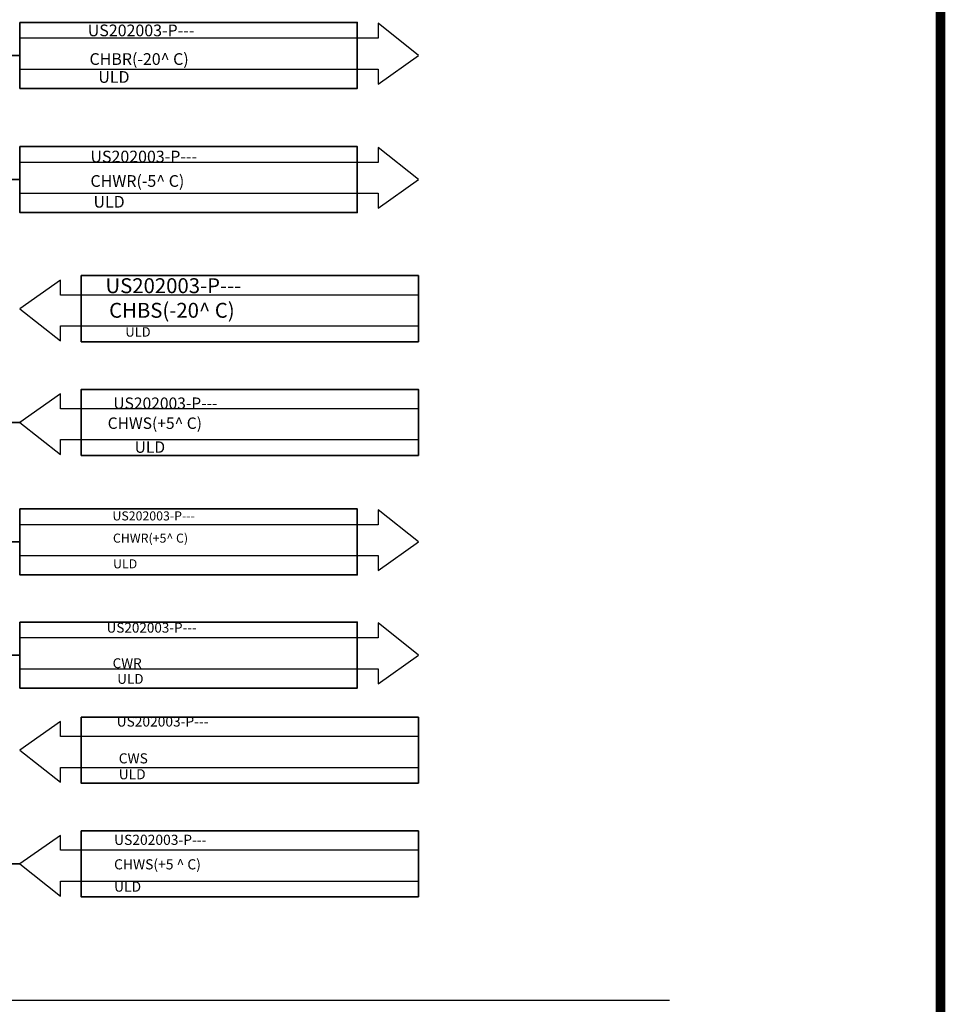
# Model space of a CAD drawing. Units: millimetres. Extents: x 353872 to 441597, y 126154 to 187356.
# Tile 27 of 28: x 426416 to 440911, y 157042 to 172470. Entities that reach past the tile are written whole.
import ezdxf

# ---------------------------------------------------------------- set-up
doc = ezdxf.new("R2010")
doc.units = ezdxf.units.MM
doc.linetypes.add('ACAD_ISO02W100', pattern=[15, 12, -3])
for name, color, linetype, lineweight in [('P-ANNO-TEXT', 7, 'Continuous', 25), ('P-ANNO-TTLB', 7, 'Continuous', 25), ('P-BNDY', 4, 'ACAD_ISO02W100', 25), ('P-EQPM', 5, 'Continuous', 35), ('P-PIPE', 3, 'Continuous', 35)]:
    doc.layers.add(name, color=color, linetype=linetype, lineweight=lineweight)
doc.styles.get("Standard").update_dxf_attribs({"font": 'arial.ttf'})

msp = doc.modelspace()

# ---------------------------------------------------------------- linework, layer by layer
at = {"layer": 'P-ANNO-TTLB', "const_width": 152.43}
msp.add_lwpolyline([(353948.03, 187280.05), (353948.03, 126916.34), (440835.19, 126916.34), (440835.19, 187280.05)], close=True, dxfattribs=at)
at = {"layer": 'P-ANNO-TTLB'}
for points in [[(426420.76, 171696.11), (432027.57, 171696.11), (432027.57, 171462.13), (432660.97, 171910.2), (432027.57, 172413.25), (432027.57, 172179.27), (426420.76, 172179.27)], [(426420.76, 169750.61), (432027.57, 169750.61), (432027.57, 169516.63), (432660.97, 169964.7), (432027.57, 170467.75), (432027.57, 170233.77), (426420.76, 170233.77)], [(432660.97, 168155.85), (427054.17, 168155.85), (427054.17, 168389.83), (426420.76, 167941.76), (427054.17, 167438.72), (427054.17, 167672.7), (432660.97, 167672.7)], [(432660.97, 166374.26), (427054.17, 166374.26), (427054.17, 166608.24), (426420.76, 166160.17), (427054.17, 165657.12), (427054.17, 165891.1), (432660.97, 165891.1)], [(426420.76, 164072.64), (432027.57, 164072.64), (432027.57, 163838.66), (432660.97, 164286.73), (432027.57, 164789.77), (432027.57, 164555.79), (426420.76, 164555.79)], [(426420.76, 162300.1), (432027.57, 162300.1), (432027.57, 162066.12), (432660.97, 162514.19), (432027.57, 163017.23), (432027.57, 162783.25), (426420.76, 162783.25)], [(432660.97, 161237.58), (427054.17, 161237.58), (427054.17, 161471.56), (426420.76, 161023.49), (427054.17, 160520.45), (427054.17, 160754.43), (432660.97, 160754.43)], [(432660.97, 159455.98), (427054.17, 159455.98), (427054.17, 159689.96), (426420.76, 159241.9), (427054.17, 158738.85), (427054.17, 158972.83), (432660.97, 158972.83)]]:
    msp.add_lwpolyline(points, dxfattribs=at)
at = {"layer": 'P-BNDY'}
msp.add_line((436591, 157104.68), (386532.91, 157104.68), dxfattribs=at)
at = {"layer": 'P-EQPM'}
for points in [[(426420.76, 172427.81), (431701.74, 172427.81), (431701.74, 171392.59), (426420.76, 171392.59)], [(426420.76, 170482.31), (431701.74, 170482.31), (431701.74, 169447.09), (426420.76, 169447.09)], [(432660.97, 167424.15), (427380, 167424.15), (427380, 168459.38), (432660.97, 168459.38)], [(432660.97, 165642.56), (427380, 165642.56), (427380, 166677.78), (432660.97, 166677.78)], [(426420.76, 164804.34), (431701.74, 164804.34), (431701.74, 163769.11), (426420.76, 163769.11)], [(426420.76, 163031.8), (431701.74, 163031.8), (431701.74, 161996.57), (426420.76, 161996.57)], [(432660.97, 160505.88), (427380, 160505.88), (427380, 161541.1), (432660.97, 161541.1)], [(432660.97, 158724.28), (427380, 158724.28), (427380, 159759.51), (432660.97, 159759.51)]]:
    msp.add_lwpolyline(points, close=True, dxfattribs=at)
at = {"layer": 'P-PIPE'}
for p, q in [((426420.76, 171910.2), (422379.04, 171907.06)), ((426420.76, 169964.7), (422379.04, 169964.7)), ((426439.3, 166160.17), (422437.83, 166160.17)), ((426420.76, 164286.73), (423379.37, 164286.73)), ((426420.76, 162514.19), (422688.58, 162514.19)), ((426420.76, 159241.9), (423545.52, 159241.9))]:
    msp.add_line(p, q, dxfattribs=at)

# ---------------------------------------------------------------- texts
at = {"layer": 'P-ANNO-TEXT'}
for s, height, p in [('US202003-P---', 183.3994, (427482.35, 172210.16)), ('CHBR(-20^  C)', 183.3994, (427509.64, 171761.64)), ('ULD', 183.399, (427647.52, 171480.84)), ('US202003-P---', 183.3994, (427524.22, 170233.77)), ('CHWR(-5^  C)', 183.3994, (427524.22, 169850.86)), ('ULD', 183.399, (427571.52, 169525.21)), ('US202003-P---', 233.6464, (427759.36, 168185.37)), ('CHBS(-20^  C)', 233.6464, (427816.34, 167799.73)), ('ULD', 148.533, (428070.7, 167503.59)), ('US202003-P---', 179.169, (427882.43, 166371.24)), ('CHWS(+5^  C)', 179.169, (427793.74, 166058.16)), ('ULD', 179.169, (428216.26, 165683.64)), ('US202003-P---', 141.7714, (427869.13, 164624.2)), ('CHWR(+5^  C)', 141.7714, (427876.59, 164275.73)), ('ULD', 141.771, (427879, 163872.87)), ('US202003-P---', 154.937, (427777.23, 162866.03)), ('CWR', 154.937, (427871.85, 162309.19)), ('ULD', 154.937, (427943.15, 162063.84)), ('US202003-P---', 158.1582, (427934.09, 161394.36)), ('CWS', 158.158, (427967.26, 160817.03)), ('ULD', 158.158, (427967.26, 160568.09)), ('US202003-P---', 158.9667, (427894.27, 159540.17)), ('CHWS(+5 ^  C)', 158.9667, (427894.27, 159156.13)), ('ULD', 158.967, (427894.27, 158807.3))]:
    msp.add_text(s, height=height, dxfattribs=at).set_placement(p)

doc.saveas('drawing.dxf')
